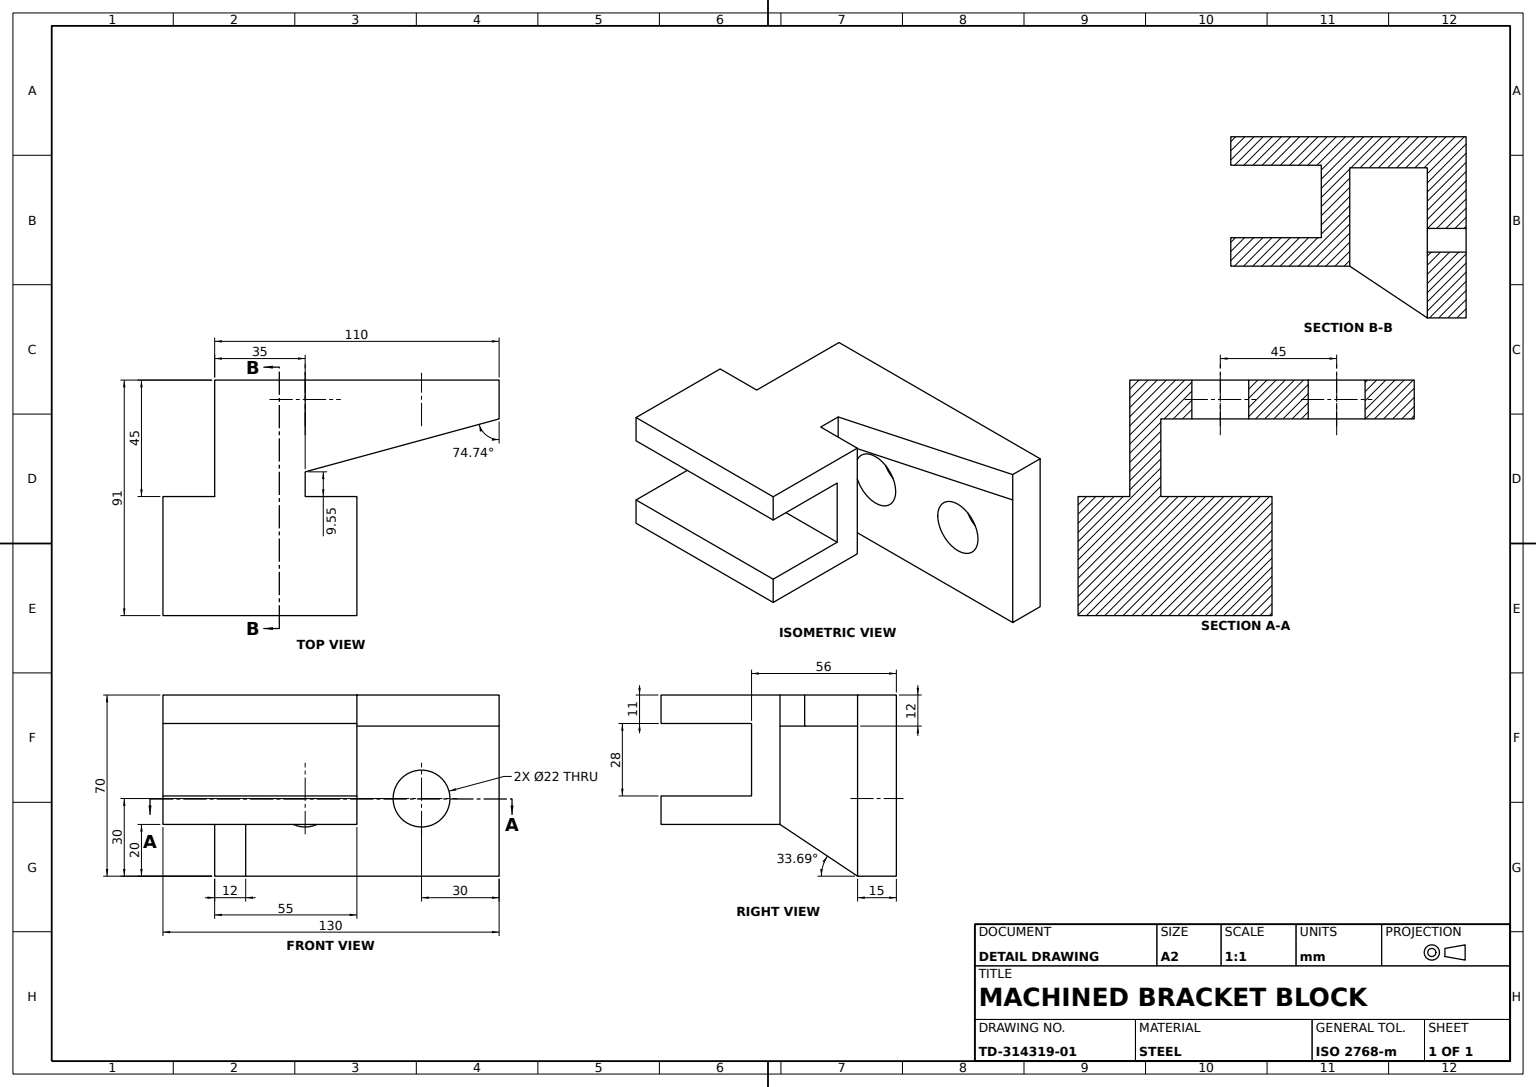
SolidWorks part; units mm, degrees
material "Plain Carbon Steel"
ref_plane "Front Plane" through (0, 0, 0) normal (0, 0, 1) x (1, 0, 0)
ref_plane "Top Plane" through (0, 0, 0) normal (0, 1, 0) x (1, 0, 0)
ref_plane "Right Plane" through (0, 0, 0) normal (1, 0, 0) x (0, 0, -1)
sketch "Base Plate Sketch" plane through (0, 0, 0) normal (0, 0, 1) x (1, 0, 0)
  line L0 (0, 0) -> (110, 0)
  line L1 (110, 0) -> (110, 70)
  line L2 (110, 70) -> (0, 70)
  line L3 (0, 70) -> (0, 0)
  dimension "D1" = 110
  dimension "D2" = 70
extrude "Base Plate 15mm" add sketch "Base Plate Sketch" along normal blind 15
sketch "Triangular Wall Sketch" plane through (0, 70, 0) normal (0, 1, 0) x (1, 0, 0)
  line L0 (0, -15) -> (0, -45)
  line L1 (0, -45) -> (110, -15)
  line L2 (110, -15) -> (0, -15)
  line L4 (110, 0) -> (0, 0) construction
  dimension "D1" = 45
extrude "Triangular Wall 12mm" add sketch "Triangular Wall Sketch" against normal blind 12
sketch "Wall Extension Sketch" plane through (0, 0, 0) normal (-1, 0, 0) x (0, 0, 1)
  line L0 (45, 58) -> (45, 20)
  line L1 (45, 20) -> (15, 0)
  line L2 (15, 0) -> (15, 58)
  line L3 (15, 58) -> (45, 58)
  line L5 (15, 0) -> (0, 0) construction
  dimension "D1" = 20
extrude "Wall Extension 12mm" add sketch "Wall Extension Sketch" against normal blind 12
sketch "Wedge Gusset Sketch" plane through (0, 70, 0) normal (0, 1, 0) x (1, 0, 0)
  line L0 (0, -45) -> (35, -45)
  line L1 (35, -45) -> (35, -35.4545)
  line L2 (0, -45) -> (110, -15) construction
  line L3 (35, -35.4545) -> (0, -45)
  line L4 (0, -45) -> (0, 0) construction
  dimension "D1" = 35
extrude "Wedge Gusset 12mm" add sketch "Wedge Gusset Sketch" against normal blind 12
sketch "Top Profile Sketch" plane through (0, 70, 0) normal (0, 1, 0) x (1, 0, 0)
  line L0 (17.5, -45) -> (55, -45)
  line L1 (0, -45) -> (35, -45) construction
  line L2 (55, -45) -> (55, -56)
  line L3 (55, -56) -> (-20, -56)
  line L4 (-20, -56) -> (-20, -45)
  line L5 (-20, -45) -> (17.5, -45)
  line L6 (0, -45) -> (0, 0) construction
  line L7 (110, 0) -> (0, 0) construction
  dimension "D1" = 55
  dimension "D2" = 56
extrude "Top Profile Boss 11mm" add sketch "Top Profile Sketch" against normal blind 11
sketch "Profile Arm Sketch" plane through (55, 0, 0) normal (1, 0, 0) x (0, 0, -1)
  line L0 (-45, 59) -> (-45, 31)
  line L1 (-45, 20) -> (-45, 58) construction
  line L2 (-56, 31) -> (-80, 31)
  line L3 (-80, 31) -> (-80, 20)
  line L4 (-80, 20) -> (-45, 20)
  line L5 (-45, 20) -> (-45, 31)
  line L6 (-56, 59) -> (-56, 31)
  line L7 (-45, 59) -> (-56, 59)
  dimension "D1" = 24
extrude "Profile Arm 75mm" add sketch "Profile Arm Sketch" against normal blind 75
sketch "Block Arm Sketch" plane through (55, 0, 0) normal (1, 0, 0) x (0, 0, -1)
  line L0 (-56, 70) -> (-80, 70)
  line L1 (-80, 70) -> (-80, 59)
  line L2 (-80, 59) -> (-56, 59)
  line L3 (-56, 31) -> (-56, 70) construction
  line L4 (-56, 59) -> (-56, 70)
  line L5 (-56, 31) -> (-80, 31) construction
  dimension "D1" = 24
  dimension "D2" = 28
extrude "Block Arm 75mm" add sketch "Block Arm Sketch" against normal blind 75
sketch "Hole Circles 2xØ22 Sketch" plane through (0, 0, 15) normal (0, 0, 1) x (1, 0, 0)
  line L0 (110, 0) -> (110, 58) construction
  line L1 (12, 0) -> (110, 0) construction
  circle A0 centre (80, 30) radius 11
  circle A1 centre (35, 30) radius 11
  dimension "D1" = 22
  dimension "D2" = 22
  dimension "D6" = 22
  dimension "D3" = 30
  dimension "D4" = 45
  dimension "D5" = 30
extrude "Holes 2xØ22" cut sketch "Hole Circles 2xØ22 Sketch" against normal blind 15
sketch "Upper Jaw Sketch" plane through (55, 0, 0) normal (1, 0, 0) x (0, 0, -1)
  line L0 (-80, 70) -> (-91, 70)
  line L1 (-91, 70) -> (-91, 59)
  line L2 (-91, 59) -> (-80, 59)
  line L3 (-80, 59) -> (-80, 70)
extrude "Upper Jaw 75mm" add sketch "Upper Jaw Sketch" against normal blind 75
sketch "Lower Jaw Sketch" plane through (55, 0, 0) normal (1, 0, 0) x (0, 0, -1)
  line L0 (-80, 31) -> (-91, 31)
  line L1 (-91, 31) -> (-91, 20)
  line L2 (-91, 20) -> (-80, 20)
  line L3 (-80, 20) -> (-80, 31)
extrude "Lower Jaw 75mm" add sketch "Lower Jaw Sketch" against normal blind 75
